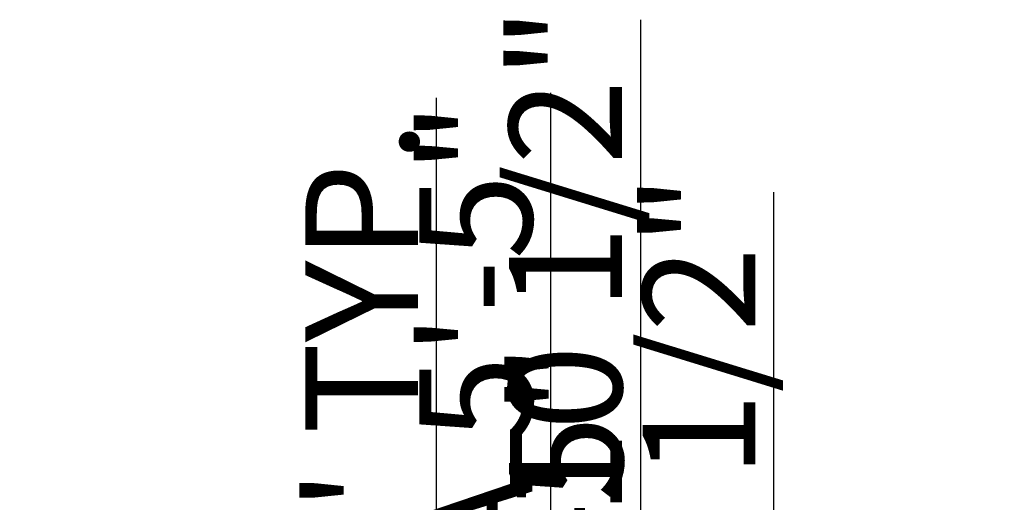
# Model space of a CAD drawing. Units: inches. Extents: x -299 to 1164, y -2 to 940.
# Tile 9 of 11: x 284 to 598, y 786 to 940. Entities that reach past the tile are written whole.
import ezdxf

# ---------------------------------------------------------------- set-up
doc = ezdxf.new("R2010")
doc.units = ezdxf.units.IN
doc.layers.add('dimensions', color=191, linetype='Continuous', lineweight=18)
doc.styles.get("Standard").update_dxf_attribs({"font": 'arial.ttf'})
doc.dimstyles.new('ISO-25', dxfattribs={"dimtxt": 36, "dimasz": 36, "dimexe": 1.25, "dimexo": 0.625, "dimtad": 1, "dimlunit": 3, "dimtxsty": 'Standard', "dimcen": 2.5, "dimazin": 0, "dimtfac": 1, "dimtmove": 0, "dimatfit": 3, "dimfxl": 1, "dimarcsym": 0})

# ---------------------------------------------------------------- blocks, each defined once
blk = doc.blocks.new('*D20')
at = {"layer": 'Defpoints', "color": 0, "transparency": 16777216}
for p in [(514.78, 631.57), (524.62, 631.57), (514.78, 602.94)]:
    blk.add_point(p, dxfattribs=at)
at = {"layer": 'dimensions', "color": 0, "lineweight": -2, "transparency": 16777216}
for p, q in [((524.62, 667.57), (524.62, 885.02)), ((515.4, 631.57), (525.87, 631.57)), ((524.62, 602.94), (524.62, 631.57)), ((515.4, 602.94), (525.87, 602.94)), ((524.62, 566.94), (524.62, 530.94))]:
    blk.add_line(p, q, dxfattribs=at)
at = {"layer": 'dimensions', "color": 0, "transparency": 16777216}
for points in [[(518.62, 667.57), (530.62, 667.57), (524.62, 631.57)], [(518.62, 566.94), (530.62, 566.94), (524.62, 602.94)]]:
    blk.add_solid(points, dxfattribs=at)
at = {"layer": 'dimensions', "color": 0, "transparency": 16777216, "insert": (505.38, 794.29), "char_height": 36, "attachment_point": 5, "rotation": 90}
blk.add_mtext('2\'-4 1/2"', dxfattribs=at)
blk = doc.blocks.new('*D25')
at = {"layer": 'Defpoints', "color": 0, "transparency": 16777216}
for p in [(443.65, 597.1), (453.38, 597.1), (443.65, 532.21)]:
    blk.add_point(p, dxfattribs=at)
at = {"layer": 'dimensions', "color": 0, "lineweight": -2, "transparency": 16777216}
for p, q in [((453.38, 633.1), (453.38, 916.77)), ((444.27, 597.1), (454.63, 597.1)), ((453.38, 532.21), (453.38, 597.1)), ((444.27, 532.21), (454.63, 532.21)), ((453.38, 496.21), (453.38, 460.21))]:
    blk.add_line(p, q, dxfattribs=at)
at = {"layer": 'dimensions', "color": 0, "transparency": 16777216}
for points in [[(447.38, 633.1), (459.38, 633.1), (453.38, 597.1)], [(447.38, 496.21), (459.38, 496.21), (453.38, 532.21)]]:
    blk.add_solid(points, dxfattribs=at)
at = {"layer": 'dimensions', "color": 0, "transparency": 16777216, "insert": (434.13, 792.94), "char_height": 36, "attachment_point": 5, "rotation": 90}
blk.add_mtext('SOFA 5\'-5"', dxfattribs=at)
blk = doc.blocks.new('*D27')
at = {"layer": 'Defpoints', "color": 0, "transparency": 16777216}
for p in [(412.07, 375.49), (416.95, 375.49), (412.07, 342.99)]:
    blk.add_point(p, dxfattribs=at)
at = {"layer": 'dimensions', "color": 0, "lineweight": -2, "transparency": 16777216}
for p, q in [((416.95, 411.49), (416.95, 915.12)), ((412.7, 375.49), (418.2, 375.49)), ((416.95, 342.99), (416.95, 375.49)), ((412.7, 342.99), (418.2, 342.99)), ((416.95, 306.99), (416.95, 270.99))]:
    blk.add_line(p, q, dxfattribs=at)
at = {"layer": 'dimensions', "color": 0, "transparency": 16777216}
for points in [[(410.95, 411.49), (422.95, 411.49), (416.95, 375.49)], [(410.95, 306.99), (422.95, 306.99), (416.95, 342.99)]]:
    blk.add_solid(points, dxfattribs=at)
at = {"layer": 'dimensions', "color": 0, "transparency": 16777216, "insert": (397.69, 681.3), "char_height": 36, "attachment_point": 5, "rotation": 90}
blk.add_mtext('DOOR 2\'-8 1/2" TYP.', dxfattribs=at)
blk = doc.blocks.new('*D63')
at = {"layer": 'Defpoints', "color": 0, "transparency": 16777216}
for p in [(658.07, 623.87), (658.07, 510.33)]:
    blk.add_point(p, dxfattribs=at)
at = {"layer": 'dimensions', "color": 0, "lineweight": -2, "transparency": 16777216}
for p, q in [((658.07, 911.15), (658.07, 659.87)), ((658.07, 510.33), (658.07, 623.87))]:
    blk.add_line(p, q, dxfattribs=at)
at = {"layer": 'dimensions', "color": 0, "transparency": 16777216}
blk.add_solid([(652.07, 659.87), (664.07, 659.87), (658.07, 623.87)], dxfattribs=at)
at = {"layer": 'dimensions', "color": 0, "transparency": 16777216, "insert": (638.83, 803.51), "char_height": 36, "attachment_point": 5, "rotation": 90}
blk.add_mtext('R9\'-5 1/2"', dxfattribs=at)
blk = doc.blocks.new('*D67')
at = {"layer": 'Defpoints', "color": 0, "transparency": 16777216}
for p in [(481.98, 624.8), (481.98, 530.15)]:
    blk.add_point(p, dxfattribs=at)
at = {"layer": 'dimensions', "color": 0, "lineweight": -2, "transparency": 16777216}
for p, q in [((481.98, 940.06), (481.98, 660.8)), ((481.98, 530.15), (481.98, 624.8))]:
    blk.add_line(p, q, dxfattribs=at)
at = {"layer": 'dimensions', "color": 0, "transparency": 16777216}
blk.add_solid([(475.98, 660.8), (487.98, 660.8), (481.98, 624.8)], dxfattribs=at)
at = {"layer": 'dimensions', "color": 0, "transparency": 16777216, "insert": (462.74, 818.43), "char_height": 36, "attachment_point": 5, "rotation": 90}
blk.add_mtext('R7\'-10 1/2"', dxfattribs=at)
blk = doc.blocks.new('*D69')
at = {"layer": 'Defpoints', "color": 0, "transparency": 16777216}
for p in [(481.98, 629.49), (481.98, 540.26)]:
    blk.add_point(p, dxfattribs=at)
at = {"layer": 'dimensions', "color": 0, "lineweight": -2, "transparency": 16777216}
for p, q in [((481.98, 832.89), (481.98, 665.49)), ((481.98, 540.26), (481.98, 629.49))]:
    blk.add_line(p, q, dxfattribs=at)
at = {"layer": 'dimensions', "color": 0, "transparency": 16777216}
blk.add_solid([(475.98, 665.49), (487.98, 665.49), (481.98, 629.49)], dxfattribs=at)
at = {"layer": 'dimensions', "color": 0, "transparency": 16777216, "insert": (463.05, 767.19), "char_height": 36, "attachment_point": 5, "rotation": 90}
blk.add_mtext('R7\'-5"', dxfattribs=at)

msp = doc.modelspace()

# ---------------------------------------------------------------- dimensions: what is measured, and where the dimension line sits
at = {"layer": 'dimensions'}
for center, mpoint, picture, middle in [((481.977, 530.151), (481.977, 624.803), '*D67', (462.738, 818.431)), ((658.071, 510.329), (658.071, 623.868), '*D63', (638.832, 803.511)), ((481.977, 540.262), (481.977, 629.489), '*D69', (463.045, 767.189))]:
    dim = msp.add_radius_dim(center=center, mpoint=mpoint, dimstyle='ISO-25', override={"dimdec": 1, "dimlfac": 1, "dimrnd": 0, "dimzin": 1, "dimdsep": 46, "dimlunit": 4, "dimfrac": 2}, dxfattribs=at)
    dim.commit()
    dim.dimension.update_dxf_attribs({"geometry": picture, "text_midpoint": middle})
for base, p1, p2, text, picture, middle in [((416.946, 375.489), (412.071, 342.989), (412.071, 375.489), 'DOOR <> TYP.', '*D27', (397.695, 681.304)), ((453.378, 597.099), (443.646, 532.214), (443.646, 597.099), 'SOFA <>', '*D25', (434.127, 792.936))]:
    dim = msp.add_linear_dim(base=base, p1=p1, p2=p2, angle=90, text=text, dimstyle='ISO-25', override={"dimdec": 1, "dimlfac": 1, "dimrnd": 0, "dimzin": 1, "dimdsep": 46, "dimlunit": 4, "dimfrac": 2}, dxfattribs=at)
    dim.commit()
    dim.dimension.update_dxf_attribs({"geometry": picture, "text_midpoint": middle})
dim = msp.add_linear_dim(base=(524.619, 631.572), p1=(514.778, 602.936), p2=(514.778, 631.572), angle=90, dimstyle='ISO-25', override={"dimdec": 1, "dimlfac": 1, "dimrnd": 0, "dimzin": 1, "dimdsep": 46, "dimlunit": 4, "dimfrac": 2}, dxfattribs=at)
dim.commit()
dim.dimension.update_dxf_attribs({"geometry": '*D20', "text_midpoint": (505.38, 794.295)})

doc.saveas('drawing.dxf')
